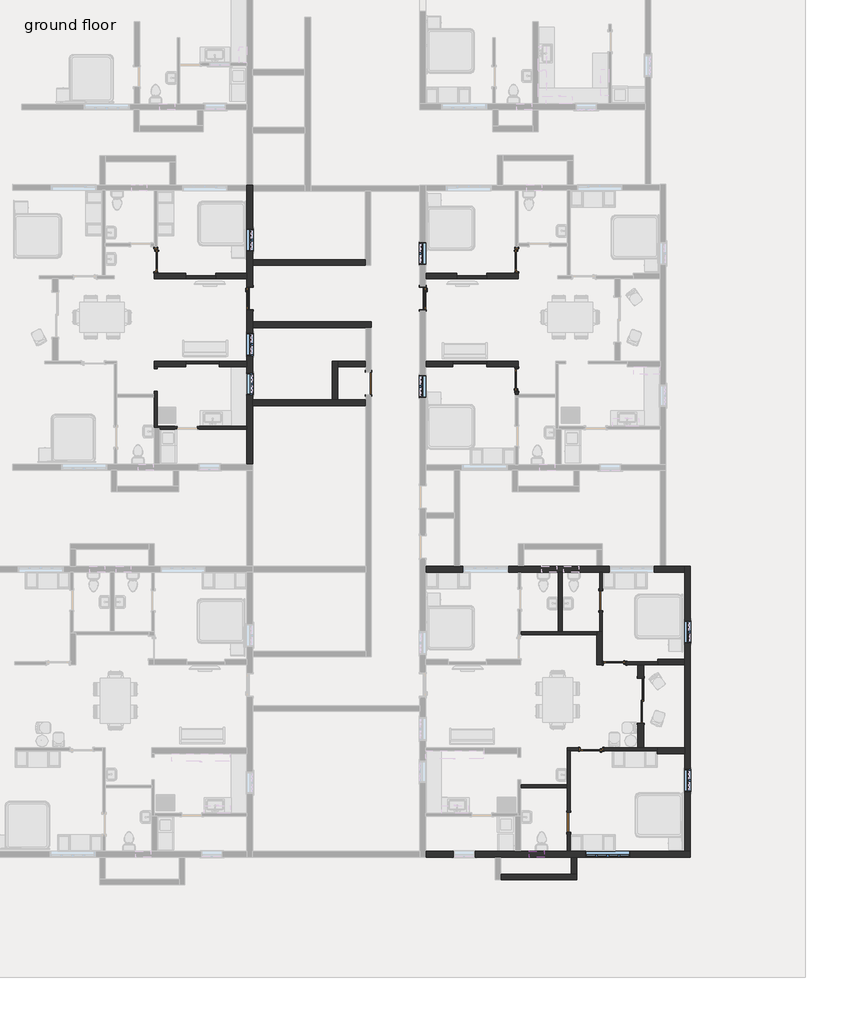
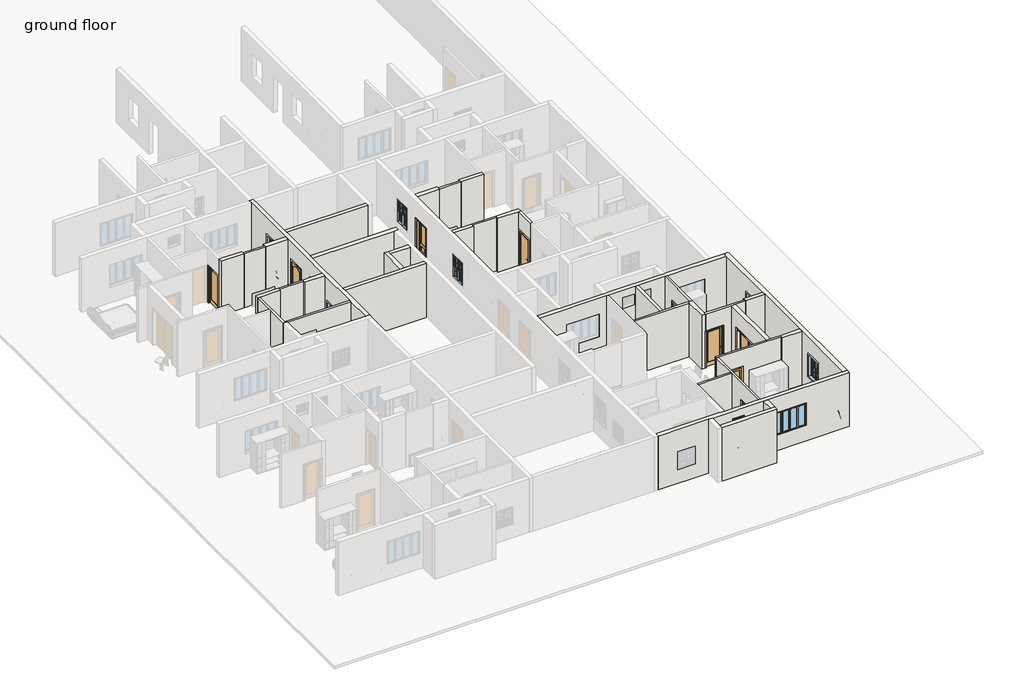
# One storey, part 3 of 16: 37 walls, 11 doors, 9 windows.
"""IFC4 building model written with IfcOpenShell, lengths in millimetres."""

from ifc_helpers import new_model, si_unit, point, frame, origin, place, context, project, spatial, polyline, ellipse_curve, trimmed, outline, extrude, faceted_brep, transform, mapped, element, save
from ifc_brep_helpers import plane_surface, extruded_surface, advanced_brep
from components import door_fe8ae985, door_f079f64e, door_d4d75d1e, door_a3feeac7, door_3c6ab76a, door_38851409, door_d141acb4, door_0ca8825f, window_ced37e8f, window_5487fb6d, window_f2d8fef0, window_45970670

model = new_model("IFC4")

# Units and contexts
model_context = context("Model", 3, world=origin())
ifc_project = project(units=[si_unit("LENGTHUNIT", "METRE", prefix="MILLI")], contexts=[model_context])

# Site, building, storey
site = spatial("IfcSite", under=ifc_project)
building = spatial("IfcBuilding", under=site)
storey = spatial("IfcBuildingStorey", under=building, Name="ground floor", Elevation=609.6)

# Doors
placement = place(None, origin())
door_shape = door_fe8ae985(model_context)
element("IfcDoor", 1, ObjectType="36\" x 84\"", at=placement, inside=storey, context=model_context, shape_type="MappedRepresentation", body=[
    mapped(door_shape, transform((59474.0062819, -2594.7113664, 609.6), x_axis=(0.0, 1.0, 0.0), y_axis=(-1.0, 0.0, 0.0), z_axis=(0.0, 0.0, 1.0))),
])
door_2_shape = door_f079f64e(model_context)
element("IfcDoor", 2, ObjectType="36\" x 84\"", at=placement, inside=storey, context=model_context, shape_type="MappedRepresentation", body=[
    mapped(door_2_shape, transform((52422.151243, -2594.7113664, 609.6), x_axis=(0.0, 1.0, 0.0), y_axis=(-1.0, 0.0, 0.0), z_axis=(0.0, 0.0, 1.0))),
])
door_3_shape = door_d4d75d1e(model_context)
element("IfcDoor", 3, ObjectType="Door-Double-Sliding : 72\" x 84\"", at=placement, inside=storey, context=model_context, shape_type="MappedRepresentation", body=[
    mapped(door_3_shape, transform((68221.1312819, -18980.3865909, 609.6), x_axis=(0.0, -1.0, 0.0), y_axis=(1.0, 0.0, 0.0), z_axis=(0.0, 0.0, 1.0))),
])
door_4_shape = door_a3feeac7(model_context)
element("IfcDoor", 4, ObjectType="Door-Interior-Single-1_Panel-Wood : 36\" x 84\"", at=placement, inside=storey, context=model_context, shape_type="MappedRepresentation", body=[
    mapped(door_4_shape, transform((63296.7062819, -1042.1363664, 609.6), x_axis=(0.0, -1.0, 0.0), y_axis=(1.0, 0.0, 0.0), z_axis=(0.0, 0.0, 1.0))),
])
element("IfcDoor", 5, ObjectType="Door-Interior-Single-1_Panel-Wood : 36\" x 84\"", at=placement, inside=storey, context=model_context, shape_type="MappedRepresentation", body=[
    mapped(door_4_shape, transform((67281.3312819, -17453.2115909, 609.6), x_axis=(-1.0, 0.0, 0.0), y_axis=(0.0, -1.0, 0.0), z_axis=(0.0, 0.0, 1.0))),
])
door_5_shape = door_3c6ab76a(model_context)
element("IfcDoor", 6, ObjectType="Door-Interior-Single-1_Panel-Wood : 36\" x 84\"", at=placement, inside=storey, context=model_context, shape_type="MappedRepresentation", body=[
    mapped(door_5_shape, transform((48599.451243, -1042.1363664, 609.6), x_axis=(0.0, -1.0, 0.0), y_axis=(1.0, 0.0, 0.0), z_axis=(0.0, 0.0, 1.0))),
])
element("IfcDoor", 7, ObjectType="Door-Interior-Single-1_Panel-Wood : 36\" x 84\"", at=placement, inside=storey, context=model_context, shape_type="MappedRepresentation", body=[
    mapped(door_5_shape, transform((63296.7062819, -5912.5863664, 609.6), x_axis=(0.0, 1.0, 0.0), y_axis=(-1.0, 0.0, 0.0), z_axis=(0.0, 0.0, 1.0))),
])
element("IfcDoor", 8, ObjectType="Door-Interior-Single-1_Panel-Wood : 36\" x 84\"", at=placement, inside=storey, context=model_context, shape_type="MappedRepresentation", body=[
    mapped(door_5_shape, transform((66335.1812819, -20964.6408586, 609.6), x_axis=(-1.0, 0.0, 0.0), y_axis=(0.0, -1.0, 0.0), z_axis=(0.0, 0.0, 1.0))),
])
door_6_shape = door_38851409(model_context)
element("IfcDoor", 9, ObjectType="Single-Flush : 32\" x 84\"", at=placement, inside=storey, context=model_context, shape_type="MappedRepresentation", body=[
    mapped(door_6_shape, transform((66728.8812819, -14903.6865909, 609.6), x_axis=(0.0, -1.0, 0.0), y_axis=(1.0, 0.0, 0.0), z_axis=(0.0, 0.0, 1.0))),
])
door_7_shape = door_d141acb4(model_context)
element("IfcDoor", 10, ObjectType="Single-Flush : 32\" x 84\"", at=placement, inside=storey, context=model_context, shape_type="MappedRepresentation", body=[
    mapped(door_7_shape, transform((65420.7812819, -23939.7365909, 609.6), x_axis=(0.0, 1.0, 0.0), y_axis=(-1.0, 0.0, 0.0), z_axis=(0.0, 0.0, 1.0))),
])
door_8_shape = door_0ca8825f(model_context)
element("IfcDoor", 11, ObjectType="Single-Flush : 36\" x 84\"", at=placement, inside=storey, context=model_context, shape_type="MappedRepresentation", body=[
    mapped(door_8_shape, transform((57261.0312819, -6052.4343195, 609.6), x_axis=(0.0, -1.0, 0.0), y_axis=(1.0, 0.0, 0.0), z_axis=(0.0, 0.0, 1.0))),
])

# Walls
element("IfcWall", 12, ObjectType="Generic - 4.5\"", at=placement, inside=storey, context=model_context, shape_type="SweptSolid", body=[
    extrude(outline(polyline([(51049.0749549, -1794.6113664), (49824.9103812, -1794.6113664), (49824.9103812, -1680.3113664), (51049.0749549, -1680.3113664), (51049.0749549, -1794.6113664)])), frame((0.0, 0.0, 609.6), z_axis=(0.0, 0.0, 1.0), x_axis=(1.0, 0.0, 0.0)), (0.0, 0.0, 1.0), 3200.4),
])
element("IfcWall", 13, ObjectType="Generic - 4.5\"", at=placement, inside=storey, context=model_context, shape_type="SweptSolid", body=[
    extrude(outline(polyline([(49809.126243, -5147.4113664), (51180.726243, -5147.4113664), (51180.726243, -5261.7113664), (49809.126243, -5261.7113664), (49809.126243, -5147.4113664)])), frame((0.0, 0.0, 609.6), z_axis=(0.0, 0.0, 1.0), x_axis=(1.0, 0.0, 0.0)), (0.0, 0.0, 1.0), 3200.4),
])
element("IfcWall", 14, ObjectType="Generic - 4.5\"", at=placement, inside=storey, context=model_context, shape_type="AdvancedBrep", body=[
    advanced_brep(
    [(48539.126243, -5376.0113664, 609.6), (48539.126243, -5455.3863664, 609.6), (48539.126243, -5455.3863664, 2540.0), (48539.126243, -6369.7863664, 2540.0), (48539.126243, -6369.7863664, 609.6), (48539.126243, -6506.3113664, 609.6), (48539.126243, -6620.6113664, 609.6), (48539.126243, -7858.8613664, 609.6), (48539.126243, -7858.8613664, 3810.0), (48539.126243, -6620.6113664, 3810.0), (48539.126243, -6506.3113664, 3810.0), (48539.126243, -5376.0113664, 3810.0), (48653.426243, -5455.3863664, 2540.0), (48653.426243, -5455.3863664, 609.6), (48653.426243, -5376.0113664, 609.6), (48653.426243, -5376.0113664, 3810.0), (48653.426243, -7801.7113664, 3810.0), (48653.426243, -7858.8613664, 3810.0), (48653.426243, -7858.8613664, 609.6), (48653.426243, -7801.7113664, 609.6), (48653.426243, -6369.7863664, 609.6), (48653.426243, -6369.7863664, 2540.0)],
    [
        (0, 1),
        (1, 2),
        (2, 3, ellipse_curve(frame((48539.126243, -5912.5863664, 2540.0), z_axis=(1.0, 0.0, 0.0), x_axis=(0.0, 1.0, 0.0)), 457.2, 203.2)),
        (3, 4),
        (4, 5),
        (5, 6),
        (6, 7),
        (7, 8),
        (8, 9),
        (9, 10),
        (10, 11),
        (11, 0),
        (12, 13),
        (13, 14),
        (14, 15),
        (15, 16),
        (16, 17),
        (17, 18),
        (18, 19),
        (19, 20),
        (20, 21),
        (21, 12, ellipse_curve(frame((48653.426243, -5912.5863664, 2540.0), z_axis=(-1.0, 0.0, 0.0), x_axis=(0.0, 1.0, 0.0)), 457.2, 203.2)),
        (13, 1),
        (0, 14),
        (18, 7),
        (4, 20),
        (17, 8),
        (15, 11),
        (2, 12),
        (21, 3),
    ],
    [
        plane_surface(frame((48539.126243, -5376.0113664, 609.6), z_axis=(-1.0, 0.0, 0.0), x_axis=(0.0, -1.0, 0.0))),
        plane_surface(frame((48653.426243, -5376.0113664, 609.6), z_axis=(1.0, 0.0, 0.0), x_axis=(0.0, 1.0, 0.0))),
        plane_surface(frame((48539.126243, -5261.7113664, 609.6), z_axis=(0.0, 0.0, -1.0), x_axis=(1.0, 0.0, 0.0))),
        plane_surface(frame((48539.126243, -7858.8613664, 609.6), z_axis=(0.0, -1.0, 0.0), x_axis=(1.0, 0.0, 0.0))),
        plane_surface(frame((48539.126243, -7858.8613664, 3810.0), z_axis=(0.0, 0.0, 1.0), x_axis=(1.0, 0.0, 0.0))),
        plane_surface(frame((48539.126243, -5376.0113664, 609.6), z_axis=(0.0, 1.0, 0.0), x_axis=(1.0, 0.0, 0.0))),
        extruded_surface(trimmed(ellipse_curve(frame((48767.726243, -5912.5863664, 2540.0), z_axis=(1.0, 0.0, 0.0), x_axis=(0.0, 1.0, 0.0)), 457.2, 203.2), [point((48767.726243, -5455.3863664, 2540.0))], [point((48767.726243, -6369.7863664, 2540.0))], True, "CARTESIAN"), (-114.29999999999563, 0.0, 0.0), 114.29999999999563),
        plane_surface(frame((48539.126243, -6369.7863664, 2540.0), z_axis=(0.0, 1.0, 0.0), x_axis=(1.0, 0.0, 0.0))),
        plane_surface(frame((48539.126243, -5455.3863664, 609.6), z_axis=(0.0, -1.0, 0.0), x_axis=(1.0, 0.0, 0.0))),
    ],
    [
        (0, [[1, 2, 3, 4, 5, 6, 7, 8, 9, 10, 11, 12]]),
        (1, [[13, 14, 15, 16, 17, 18, 19, 20, 21, 22]]),
        (2, [[-14, 23, -1, 24]]),
        (2, [[-20, -19, 25, -7, -6, -5, 26]]),
        (3, [[-8, -25, -18, 27]]),
        (4, [[-11, -10, -9, -27, -17, -16, 28]]),
        (5, [[-12, -28, -15, -24]]),
        (6, [[-3, 29, -22, 30]]),
        (7, [[-4, -30, -21, -26]]),
        (8, [[-2, -23, -13, -29]]),
    ],
),
])
element("IfcWall", 15, ObjectType="Generic - 4.5\"", at=placement, inside=storey, context=model_context, shape_type="Brep", body=[
    faceted_brep([(48767.726243, -7916.0113664, 609.6), (49466.226243, -7916.0113664, 609.6), (49466.226243, -7916.0113664, 2743.2), (50279.026243, -7916.0113664, 2743.2), (50279.026243, -7916.0113664, 609.6), (52311.026243, -7916.0113664, 609.6), (52311.026243, -7916.0113664, 3810.0), (48767.726243, -7916.0113664, 3810.0), (49466.226243, -7801.7113664, 2743.2), (49466.226243, -7801.7113664, 609.6), (48653.426243, -7801.7113664, 609.6), (48653.426243, -7801.7113664, 3810.0), (52311.026243, -7801.7113664, 3810.0), (52311.026243, -7801.7113664, 609.6), (50279.026243, -7801.7113664, 609.6), (50279.026243, -7801.7113664, 2743.2), (48767.726243, -7858.8613664, 609.6), (48653.426243, -7858.8613664, 609.6), (48653.426243, -7858.8613664, 3810.0), (48767.726243, -7858.8613664, 3810.0)], [[[0, 1, 2, 3, 4, 5, 6, 7]], [[8, 9, 10, 11, 12, 13, 14, 15]], [[14, 13, 5, 4]], [[10, 9, 1, 0, 16, 17]], [[7, 6, 12, 11, 18, 19]], [[0, 7, 19, 16]], [[19, 18, 17, 16]], [[18, 11, 10, 17]], [[6, 5, 13, 12]], [[2, 1, 9, 8]], [[3, 2, 8, 15]], [[4, 3, 15, 14]]]),
])
element("IfcWall", 16, ObjectType="Generic - 4.5\"", at=placement, inside=storey, context=model_context, shape_type="SweptSolid", body=[
    extrude(outline(polyline([(62071.2471437, -1794.6113664), (60847.08257, -1794.6113664), (60847.08257, -1680.3113664), (62071.2471437, -1680.3113664), (62071.2471437, -1794.6113664)])), frame((0.0, 0.0, 609.6), z_axis=(0.0, 0.0, 1.0), x_axis=(1.0, 0.0, 0.0)), (0.0, 0.0, 1.0), 3200.4),
])
element("IfcWall", 17, ObjectType="Generic - 4.5\"", at=placement, inside=storey, context=model_context, shape_type="SweptSolid", body=[
    extrude(outline(polyline([(60702.7312819, -5147.4113664), (62074.3312819, -5147.4113664), (62074.3312819, -5261.7113664), (60702.7312819, -5261.7113664), (60702.7312819, -5147.4113664)])), frame((0.0, 0.0, 609.6), z_axis=(0.0, 0.0, 1.0), x_axis=(1.0, 0.0, 0.0)), (0.0, 0.0, 1.0), 3200.4),
])
element("IfcWall", 18, ObjectType="Generic - 4.5\"", at=placement, inside=storey, context=model_context, shape_type="Brep", body=[
    faceted_brep([(66786.0312819, -17399.2365909, 3810.0), (69046.6312819, -17399.2365909, 3810.0), (69046.6312819, -17399.2365909, 609.6), (67763.9312819, -17399.2365909, 609.6), (67763.9312819, -17399.2365909, 2768.6), (66798.7312819, -17399.2365909, 2768.6), (66798.7312819, -17399.2365909, 609.6), (66786.0312819, -17399.2365909, 609.6), (69046.6312819, -17513.5365909, 3810.0), (68462.4312819, -17513.5365909, 3810.0), (68233.8312819, -17513.5365909, 3810.0), (66786.0312819, -17513.5365909, 3810.0), (66786.0312819, -17513.5365909, 609.6), (66798.7312819, -17513.5365909, 609.6), (66798.7312819, -17513.5365909, 2768.6), (67763.9312819, -17513.5365909, 2768.6), (67763.9312819, -17513.5365909, 609.6), (68233.8312819, -17513.5365909, 609.6), (68462.4312819, -17513.5365909, 609.6), (69046.6312819, -17513.5365909, 609.6)], [[[0, 1, 2, 3, 4, 5, 6, 7]], [[8, 9, 10, 11, 12, 13, 14, 15, 16, 17, 18, 19]], [[2, 19, 18, 17, 16, 3]], [[12, 7, 6, 13]], [[1, 0, 11, 10, 9, 8]], [[2, 1, 8, 19]], [[0, 7, 12, 11]], [[5, 14, 13, 6]], [[14, 5, 4, 15]], [[15, 4, 3, 16]]]),
])
element("IfcWall", 19, ObjectType="Generic - 4.5\"", at=placement, inside=storey, context=model_context, shape_type="Brep", body=[
    faceted_brep([(65363.6312819, -20904.3158586, 3810.0), (68233.8312819, -20904.3158586, 3810.0), (68462.4312819, -20904.3158586, 3810.0), (69021.2312819, -20904.3158586, 3810.0), (69021.2312819, -20904.3158586, 609.6), (68462.4312819, -20904.3158586, 609.6), (68233.8312819, -20904.3158586, 609.6), (66817.7812819, -20904.3158586, 609.6), (66817.7812819, -20904.3158586, 2768.6), (65852.5812819, -20904.3158586, 2768.6), (65852.5812819, -20904.3158586, 609.6), (65363.6312819, -20904.3158586, 609.6), (69021.2312819, -21018.6158586, 3810.0), (65477.9312819, -21018.6158586, 3810.0), (65363.6312819, -21018.6158586, 3810.0), (65363.6312819, -21018.6158586, 609.6), (65477.9312819, -21018.6158586, 609.6), (65852.5812819, -21018.6158586, 609.6), (65852.5812819, -21018.6158586, 2768.6), (66817.7812819, -21018.6158586, 2768.6), (66817.7812819, -21018.6158586, 609.6), (69021.2312819, -21018.6158586, 609.6)], [[[0, 1, 2, 3, 4, 5, 6, 7, 8, 9, 10, 11]], [[12, 13, 14, 15, 16, 17, 18, 19, 20, 21]], [[4, 21, 20, 7, 6, 5]], [[15, 11, 10, 17, 16]], [[3, 2, 1, 0, 14, 13, 12]], [[4, 3, 12, 21]], [[0, 11, 15, 14]], [[9, 18, 17, 10]], [[18, 9, 8, 19]], [[19, 8, 7, 20]]]),
])
element("IfcWall", 20, ObjectType="Generic - 4.5\"", at=placement, inside=storey, context=model_context, shape_type="Brep", body=[
    faceted_brep([(65363.6312819, -21018.6158586, 609.6), (65363.6312819, -22413.9790776, 609.6), (65363.6312819, -22528.2790776, 609.6), (65363.6312819, -23533.3365909, 609.6), (65363.6312819, -23533.3365909, 2743.2), (65363.6312819, -24346.1365909, 2743.2), (65363.6312819, -24346.1365909, 609.6), (65363.6312819, -25120.8365909, 609.6), (65363.6312819, -25120.8365909, 3810.0), (65363.6312819, -22528.2790776, 3810.0), (65363.6312819, -22413.9790776, 3810.0), (65363.6312819, -21018.6158586, 3810.0), (65477.9312819, -23533.3365909, 2743.2), (65477.9312819, -23533.3365909, 609.6), (65477.9312819, -21018.6158586, 609.6), (65477.9312819, -21018.6158586, 3810.0), (65477.9312819, -25120.8365909, 3810.0), (65477.9312819, -25120.8365909, 609.6), (65477.9312819, -24346.1365909, 609.6), (65477.9312819, -24346.1365909, 2743.2)], [[[0, 1, 2, 3, 4, 5, 6, 7, 8, 9, 10, 11]], [[12, 13, 14, 15, 16, 17, 18, 19]], [[18, 17, 7, 6]], [[14, 13, 3, 2, 1, 0]], [[11, 10, 9, 8, 16, 15]], [[0, 11, 15, 14]], [[8, 7, 17, 16]], [[4, 3, 13, 12]], [[5, 4, 12, 19]], [[6, 5, 19, 18]]]),
])
element("IfcWall", 21, ObjectType="Generic - 4.5\"", at=placement, inside=storey, context=model_context, shape_type="SweptSolid", body=[
    extrude(outline(polyline([(63458.6312819, -22413.9790776), (65363.6312819, -22413.9790776), (65363.6312819, -22528.2790776), (63458.6312819, -22528.2790776), (63458.6312819, -22413.9790776)])), frame((0.0, 0.0, 609.6), z_axis=(0.0, 0.0, 1.0), x_axis=(1.0, 0.0, 0.0)), (0.0, 0.0, 1.0), 3200.4),
])
element("IfcWall", 22, ObjectType="Generic - 4.5\"", at=placement, inside=storey, context=model_context, shape_type="Brep", body=[
    faceted_brep([(63471.3312819, -16294.3365909, 609.6), (66557.4312819, -16294.3365909, 609.6), (66557.4312819, -16294.3365909, 3810.0), (63471.3312819, -16294.3365909, 3810.0), (63471.3312819, -16180.0365909, 609.6), (63471.3312819, -16180.0365909, 3810.0), (64995.3312819, -16180.0365909, 3810.0), (65147.7312819, -16180.0365909, 3810.0), (66557.4312819, -16180.0365909, 3810.0), (66557.4312819, -16180.0365909, 609.6), (65147.7312819, -16180.0365909, 609.6), (64995.3312819, -16180.0365909, 609.6)], [[[0, 1, 2, 3]], [[4, 5, 6, 7, 8, 9, 10, 11]], [[1, 0, 4, 11, 10, 9]], [[3, 2, 8, 7, 6, 5]], [[2, 1, 9, 8]], [[0, 3, 5, 4]]]),
])
element("IfcWall", 23, ObjectType="Generic - 4.5\"", at=placement, inside=storey, context=model_context, shape_type="SweptSolid", body=[
    extrude(outline(polyline([(-15310.0865909, 2743.2), (-15310.0865909, 609.6), (-16180.0365909, 609.6), (-16180.0365909, 3810.0), (-13741.6365909, 3810.0), (-13741.6365909, 609.6), (-14497.2865909, 609.6), (-14497.2865909, 2743.2), (-15310.0865909, 2743.2)])), frame((66671.7312819, 0.0, 0.0), z_axis=(1.0, 0.0, 0.0), x_axis=(0.0, 1.0, 0.0)), (0.0, 0.0, 1.0), 114.3),
])
element("IfcWall", 24, ObjectType="Generic - 4.5\"", at=placement, inside=storey, context=model_context, shape_type="SweptSolid", body=[
    extrude(outline(polyline([(-6506.3113664, 3810.0), (-5376.0113664, 3810.0), (-5376.0113664, 609.6), (-5429.9863664, 609.6), (-5429.9863664, 2768.6), (-6395.1863664, 2768.6), (-6395.1863664, 609.6), (-6506.3113664, 609.6), (-6506.3113664, 3810.0)])), frame((63242.7312819, 0.0, 0.0), z_axis=(1.0, 0.0, 0.0), x_axis=(0.0, 1.0, 0.0)), (0.0, 0.0, 1.0), 114.3),
])
element("IfcWall", 25, ObjectType="Generic - 6\"", at=placement, inside=storey, context=model_context, shape_type="SweptSolid", body=[
    extrude(outline(polyline([(64995.3312819, -16180.0365909), (64995.3312819, -13741.6365909), (65147.7312819, -13741.6365909), (65147.7312819, -16180.0365909), (64995.3312819, -16180.0365909)])), frame((0.0, 0.0, 609.6), z_axis=(0.0, 0.0, 1.0), x_axis=(1.0, 0.0, 0.0)), (0.0, 0.0, 1.0), 3200.4),
])
element("IfcWall", 26, ObjectType="Generic - 9\"", at=placement, inside=storey, context=model_context, shape_type="Brep", body=[
    faceted_brep([(52539.626243, 2007.0575277, 3810.0), (52539.626243, 2006.2512916, 3810.0), (52539.626243, 1777.6512916, 3810.0), (52539.626243, -1024.9409315, 3810.0), (52539.626243, -1253.5409315, 3810.0), (52539.626243, -3551.5389812, 3810.0), (52539.626243, -3780.1389812, 3810.0), (52539.626243, -6728.8572725, 3810.0), (52539.626243, -6957.4572725, 3810.0), (52539.626243, -9357.7253443, 3810.0), (52539.626243, -9357.7253443, 609.6), (52539.626243, -6957.4572725, 609.6), (52539.626243, -6728.8572725, 609.6), (52539.626243, -3780.1389812, 609.6), (52539.626243, -3551.5389812, 609.6), (52539.626243, -3077.3113664, 609.6), (52539.626243, -3077.3113664, 2768.6), (52539.626243, -2112.1113664, 2768.6), (52539.626243, -2112.1113664, 609.6), (52539.626243, -1253.5409315, 609.6), (52539.626243, -1024.9409315, 609.6), (52539.626243, 1777.6512916, 609.6), (52539.626243, 2006.2512916, 609.6), (52539.626243, 2007.0575277, 609.6), (52539.626243, -6512.9572725, 2438.4), (52539.626243, -5649.3572725, 2438.4), (52539.626243, -5649.3572725, 1524.0), (52539.626243, -6512.9572725, 1524.0), (52539.626243, -4006.5751738, 2844.8), (52539.626243, -4006.5751738, 1524.0), (52539.626243, -4920.9751738, 1524.0), (52539.626243, -4920.9751738, 2844.8), (52539.626243, 232.3590685, 2844.8), (52539.626243, 232.3590685, 1524.0), (52539.626243, -682.0409315, 1524.0), (52539.626243, -682.0409315, 2844.8), (52311.026243, -9357.7253443, 3810.0), (52311.026243, -7916.0113664, 3810.0), (52311.026243, -7801.7113664, 3810.0), (52311.026243, -5376.0113664, 3810.0), (52311.026243, -5147.4113664, 3810.0), (52311.026243, -1794.6113664, 3810.0), (52311.026243, -1566.0113664, 3810.0), (52311.026243, 1779.3652466, 3810.0), (52311.026243, 2007.967056, 3810.0), (52311.026243, 2007.967056, 609.6), (52311.026243, 1779.3652466, 609.6), (52311.026243, -1566.0113664, 609.6), (52311.026243, -1794.6113664, 609.6), (52311.026243, -2112.1113664, 609.6), (52311.026243, -2112.1113664, 2768.6), (52311.026243, -3077.3113664, 2768.6), (52311.026243, -3077.3113664, 609.6), (52311.026243, -5147.4113664, 609.6), (52311.026243, -5376.0113664, 609.6), (52311.026243, -7801.7113664, 609.6), (52311.026243, -7916.0113664, 609.6), (52311.026243, -9357.7253443, 609.6), (52311.026243, -6512.9572725, 2438.4), (52311.026243, -6512.9572725, 1524.0), (52311.026243, -5649.3572725, 1524.0), (52311.026243, -5649.3572725, 2438.4), (52311.026243, -4006.5751738, 2844.8), (52311.026243, -4920.9751738, 2844.8), (52311.026243, -4920.9751738, 1524.0), (52311.026243, -4006.5751738, 1524.0), (52311.026243, 232.3590685, 2844.8), (52311.026243, -682.0409315, 2844.8), (52311.026243, -682.0409315, 1524.0), (52311.026243, 232.3590685, 1524.0)], [[[0, 1, 2, 3, 4, 5, 6, 7, 8, 9, 10, 11, 12, 13, 14, 15, 16, 17, 18, 19, 20, 21, 22, 23], [24, 25, 26, 27], [28, 29, 30, 31], [32, 33, 34, 35]], [[36, 37, 38, 39, 40, 41, 42, 43, 44, 45, 46, 47, 48, 49, 50, 51, 52, 53, 54, 55, 56, 57], [58, 59, 60, 61], [62, 63, 64, 65], [66, 67, 68, 69]], [[10, 57, 56, 55, 54, 53, 52, 15, 14, 13, 12, 11]], [[45, 23, 22, 21, 20, 19, 18, 49, 48, 47, 46]], [[9, 8, 7, 6, 5, 4, 3, 2, 1, 0, 44, 43, 42, 41, 40, 39, 38, 37, 36]], [[10, 9, 36, 57]], [[0, 23, 45, 44]], [[17, 50, 49, 18]], [[50, 17, 16, 51]], [[51, 16, 15, 52]], [[59, 58, 24, 27]], [[60, 59, 27, 26]], [[61, 60, 26, 25]], [[58, 61, 25, 24]], [[29, 28, 62, 65]], [[30, 29, 65, 64]], [[31, 30, 64, 63]], [[28, 31, 63, 62]], [[33, 32, 66, 69]], [[34, 33, 69, 68]], [[35, 34, 68, 67]], [[32, 35, 67, 66]]]),
])
element("IfcWall", 27, ObjectType="Generic - 9\"", at=placement, inside=storey, context=model_context, shape_type="Brep", body=[
    faceted_brep([(48539.126243, -5376.0113664, 609.6), (48653.426243, -5376.0113664, 609.6), (49809.126243, -5376.0113664, 609.6), (49809.126243, -5376.0113664, 3810.0), (48653.426243, -5376.0113664, 3810.0), (48539.126243, -5376.0113664, 3810.0), (48539.126243, -5147.4113664, 609.6), (48539.126243, -5147.4113664, 3810.0), (49809.126243, -5147.4113664, 3810.0), (49809.126243, -5147.4113664, 609.6), (49809.126243, -5261.7113664, 609.6), (49809.126243, -5261.7113664, 3810.0)], [[[0, 1, 2, 3, 4, 5]], [[6, 7, 8, 9]], [[2, 1, 0, 6, 9, 10]], [[3, 2, 10, 9, 8, 11]], [[5, 4, 3, 11, 8, 7]], [[0, 5, 7, 6]]]),
])
element("IfcWall", 28, ObjectType="Generic - 9\"", at=placement, inside=storey, context=model_context, shape_type="Brep", body=[
    faceted_brep([(51180.726243, -5376.0113664, 609.6), (52311.026243, -5376.0113664, 609.6), (52311.026243, -5376.0113664, 3810.0), (51180.726243, -5376.0113664, 3810.0), (51180.726243, -5147.4113664, 609.6), (51180.726243, -5147.4113664, 3810.0), (52311.026243, -5147.4113664, 3810.0), (52311.026243, -5147.4113664, 609.6), (51180.726243, -5261.7113664, 609.6), (51180.726243, -5261.7113664, 3810.0)], [[[0, 1, 2, 3]], [[4, 5, 6, 7]], [[1, 0, 8, 4, 7]], [[3, 2, 6, 5, 9]], [[0, 3, 9, 5, 4, 8]], [[2, 1, 7, 6]]]),
])
element("IfcWall", 29, ObjectType="Generic - 9\"", at=placement, inside=storey, context=model_context, shape_type="Brep", body=[
    faceted_brep([(48539.126243, -1794.6113664, 609.6), (49824.9103812, -1794.6113664, 609.6), (49824.9103812, -1794.6113664, 3810.0), (48539.126243, -1794.6113664, 3810.0), (48539.126243, -1566.0113664, 609.6), (48539.126243, -1566.0113664, 3810.0), (48653.426243, -1566.0113664, 3810.0), (49824.9103812, -1566.0113664, 3810.0), (49824.9103812, -1566.0113664, 609.6), (48653.426243, -1566.0113664, 609.6), (49824.9103812, -1680.3113664, 609.6), (49824.9103812, -1680.3113664, 3810.0)], [[[0, 1, 2, 3]], [[4, 5, 6, 7, 8, 9]], [[1, 0, 4, 9, 8, 10]], [[2, 1, 10, 8, 7, 11]], [[3, 2, 11, 7, 6, 5]], [[0, 3, 5, 4]]]),
])
element("IfcWall", 30, ObjectType="Generic - 9\"", at=placement, inside=storey, context=model_context, shape_type="Brep", body=[
    faceted_brep([(51049.0749549, -1794.6113664, 609.6), (52311.026243, -1794.6113664, 609.6), (52311.026243, -1794.6113664, 3810.0), (51049.0749549, -1794.6113664, 3810.0), (51049.0749549, -1566.0113664, 609.6), (51049.0749549, -1566.0113664, 3810.0), (52311.026243, -1566.0113664, 3810.0), (52311.026243, -1566.0113664, 609.6), (51049.0749549, -1680.3113664, 609.6), (51049.0749549, -1680.3113664, 3810.0)], [[[0, 1, 2, 3]], [[4, 5, 6, 7]], [[1, 0, 8, 4, 7]], [[3, 2, 6, 5, 9]], [[0, 3, 9, 5, 4, 8]], [[2, 1, 7, 6]]]),
])
element("IfcWall", 31, ObjectType="Generic - 9\"", at=placement, inside=storey, context=model_context, shape_type="Brep", body=[
    faceted_brep([(62071.2471437, -1794.6113664, 609.6), (63357.0312819, -1794.6113664, 609.6), (63357.0312819, -1794.6113664, 3810.0), (62071.2471437, -1794.6113664, 3810.0), (62071.2471437, -1566.0113664, 609.6), (62071.2471437, -1566.0113664, 3810.0), (63242.7312819, -1566.0113664, 3810.0), (63357.0312819, -1566.0113664, 3810.0), (63357.0312819, -1566.0113664, 609.6), (63242.7312819, -1566.0113664, 609.6), (62071.2471437, -1680.3113664, 609.6), (62071.2471437, -1680.3113664, 3810.0)], [[[0, 1, 2, 3]], [[4, 5, 6, 7, 8, 9]], [[1, 0, 10, 4, 9, 8]], [[3, 2, 7, 6, 5, 11]], [[0, 3, 11, 5, 4, 10]], [[2, 1, 8, 7]]]),
])
element("IfcWall", 32, ObjectType="Generic - 9\"", at=placement, inside=storey, context=model_context, shape_type="Brep", body=[
    faceted_brep([(59585.1312819, -1794.6113664, 609.6), (60847.08257, -1794.6113664, 609.6), (60847.08257, -1794.6113664, 3810.0), (59585.1312819, -1794.6113664, 3810.0), (59585.1312819, -1566.0113664, 609.6), (59585.1312819, -1566.0113664, 3810.0), (60847.08257, -1566.0113664, 3810.0), (60847.08257, -1566.0113664, 609.6), (60847.08257, -1680.3113664, 609.6), (60847.08257, -1680.3113664, 3810.0)], [[[0, 1, 2, 3]], [[4, 5, 6, 7]], [[1, 0, 4, 7, 8]], [[2, 1, 8, 7, 6, 9]], [[3, 2, 9, 6, 5]], [[0, 3, 5, 4]]]),
])
element("IfcWall", 33, ObjectType="Generic - 9\"", at=placement, inside=storey, context=model_context, shape_type="Brep", body=[
    faceted_brep([(59585.1312819, -5376.0113664, 609.6), (60702.7312819, -5376.0113664, 609.6), (60702.7312819, -5376.0113664, 3810.0), (59585.1312819, -5376.0113664, 3810.0), (59585.1312819, -5147.4113664, 609.6), (59585.1312819, -5147.4113664, 3810.0), (60702.7312819, -5147.4113664, 3810.0), (60702.7312819, -5147.4113664, 609.6), (60702.7312819, -5261.7113664, 609.6), (60702.7312819, -5261.7113664, 3810.0)], [[[0, 1, 2, 3]], [[4, 5, 6, 7]], [[1, 0, 4, 7, 8]], [[2, 1, 8, 7, 6, 9]], [[3, 2, 9, 6, 5]], [[0, 3, 5, 4]]]),
])
element("IfcWall", 34, ObjectType="Generic - 9\"", at=placement, inside=storey, context=model_context, shape_type="Brep", body=[
    faceted_brep([(62074.3312819, -5376.0113664, 609.6), (63242.7312819, -5376.0113664, 609.6), (63357.0312819, -5376.0113664, 609.6), (63357.0312819, -5376.0113664, 3810.0), (63242.7312819, -5376.0113664, 3810.0), (62074.3312819, -5376.0113664, 3810.0), (62074.3312819, -5147.4113664, 609.6), (62074.3312819, -5147.4113664, 3810.0), (63357.0312819, -5147.4113664, 3810.0), (63357.0312819, -5147.4113664, 609.6), (62074.3312819, -5261.7113664, 609.6), (62074.3312819, -5261.7113664, 3810.0)], [[[0, 1, 2, 3, 4, 5]], [[6, 7, 8, 9]], [[2, 1, 0, 10, 6, 9]], [[5, 4, 3, 8, 7, 11]], [[0, 5, 11, 7, 6, 10]], [[3, 2, 9, 8]]]),
])
element("IfcWall", 35, ObjectType="Generic - 9\"", at=placement, inside=storey, context=model_context, shape_type="Brep", body=[
    faceted_brep([(59585.1312819, -25349.4365909, 609.6), (62419.2921849, -25349.4365909, 609.6), (62647.8921849, -25349.4365909, 609.6), (65521.3932249, -25349.4365909, 609.6), (65749.9932249, -25349.4365909, 609.6), (70367.4312819, -25349.4365909, 609.6), (70367.4312819, -25349.4365909, 3810.0), (65749.9932249, -25349.4365909, 3810.0), (65521.3932249, -25349.4365909, 3810.0), (62647.8921849, -25349.4365909, 3810.0), (62419.2921849, -25349.4365909, 3810.0), (59585.1312819, -25349.4365909, 3810.0), (66092.8932249, -25349.4365909, 2870.2), (67921.6932249, -25349.4365909, 2870.2), (67921.6932249, -25349.4365909, 1524.0), (66092.8932249, -25349.4365909, 1524.0), (60730.1921849, -25349.4365909, 2438.4), (61593.7921849, -25349.4365909, 2438.4), (61593.7921849, -25349.4365909, 1524.0), (60730.1921849, -25349.4365909, 1524.0), (64411.1312819, -25349.4365909, 3352.8), (64411.1312819, -25349.4365909, 2743.2), (63801.5312819, -25349.4365909, 2743.2), (63801.5312819, -25349.4365909, 3352.8), (59585.1312819, -25120.8365909, 609.6), (59585.1312819, -25120.8365909, 3810.0), (63230.0312819, -25120.8365909, 3810.0), (63458.6312819, -25120.8365909, 3810.0), (65363.6312819, -25120.8365909, 3810.0), (65477.9312819, -25120.8365909, 3810.0), (70138.8312819, -25120.8365909, 3810.0), (70367.4312819, -25120.8365909, 3810.0), (70367.4312819, -25120.8365909, 609.6), (70138.8312819, -25120.8365909, 609.6), (65477.9312819, -25120.8365909, 609.6), (65363.6312819, -25120.8365909, 609.6), (63458.6312819, -25120.8365909, 609.6), (63230.0312819, -25120.8365909, 609.6), (66092.8932249, -25120.8365909, 2870.2), (66092.8932249, -25120.8365909, 1524.0), (67921.6932249, -25120.8365909, 1524.0), (67921.6932249, -25120.8365909, 2870.2), (60730.1921849, -25120.8365909, 2438.4), (60730.1921849, -25120.8365909, 1524.0), (61593.7921849, -25120.8365909, 1524.0), (61593.7921849, -25120.8365909, 2438.4), (64411.1312819, -25120.8365909, 3352.8), (63801.5312819, -25120.8365909, 3352.8), (63801.5312819, -25120.8365909, 2743.2), (64411.1312819, -25120.8365909, 2743.2)], [[[0, 1, 2, 3, 4, 5, 6, 7, 8, 9, 10, 11], [12, 13, 14, 15], [16, 17, 18, 19], [20, 21, 22, 23]], [[24, 25, 26, 27, 28, 29, 30, 31, 32, 33, 34, 35, 36, 37], [38, 39, 40, 41], [42, 43, 44, 45], [46, 47, 48, 49]], [[5, 4, 3, 2, 1, 0, 24, 37, 36, 35, 34, 33, 32]], [[11, 10, 9, 8, 7, 6, 31, 30, 29, 28, 27, 26, 25]], [[0, 11, 25, 24]], [[6, 5, 32, 31]], [[39, 38, 12, 15]], [[40, 39, 15, 14]], [[41, 40, 14, 13]], [[38, 41, 13, 12]], [[43, 42, 16, 19]], [[44, 43, 19, 18]], [[45, 44, 18, 17]], [[42, 45, 17, 16]], [[21, 20, 46, 49]], [[22, 21, 49, 48]], [[23, 22, 48, 47]], [[20, 23, 47, 46]]]),
])
element("IfcWall", 36, ObjectType="Generic - 9\"", at=placement, inside=storey, context=model_context, shape_type="Brep", body=[
    faceted_brep([(70367.4312819, -25120.8365909, 609.6), (70367.4312819, -13513.0365909, 609.6), (70367.4312819, -13513.0365909, 3810.0), (70367.4312819, -25120.8365909, 3810.0), (70367.4312819, -21780.6158586, 2844.8), (70367.4312819, -21780.6158586, 1524.0), (70367.4312819, -22695.0158586, 1524.0), (70367.4312819, -22695.0158586, 2844.8), (70367.4312819, -15722.8365909, 2844.8), (70367.4312819, -15722.8365909, 1524.0), (70367.4312819, -16637.2365909, 1524.0), (70367.4312819, -16637.2365909, 2844.8), (70138.8312819, -25120.8365909, 609.6), (70138.8312819, -25120.8365909, 3810.0), (70138.8312819, -21132.9158586, 3810.0), (70138.8312819, -20904.3158586, 3810.0), (70138.8312819, -17513.5365909, 3810.0), (70138.8312819, -17284.9365909, 3810.0), (70138.8312819, -13741.6365909, 3810.0), (70138.8312819, -13513.0365909, 3810.0), (70138.8312819, -13513.0365909, 609.6), (70138.8312819, -13741.6365909, 609.6), (70138.8312819, -17284.9365909, 609.6), (70138.8312819, -17513.5365909, 609.6), (70138.8312819, -20904.3158586, 609.6), (70138.8312819, -21132.9158586, 609.6), (70138.8312819, -21780.6158586, 2844.8), (70138.8312819, -22695.0158586, 2844.8), (70138.8312819, -22695.0158586, 1524.0), (70138.8312819, -21780.6158586, 1524.0), (70138.8312819, -15722.8365909, 2844.8), (70138.8312819, -16637.2365909, 2844.8), (70138.8312819, -16637.2365909, 1524.0), (70138.8312819, -15722.8365909, 1524.0)], [[[0, 1, 2, 3], [4, 5, 6, 7], [8, 9, 10, 11]], [[12, 13, 14, 15, 16, 17, 18, 19, 20, 21, 22, 23, 24, 25], [26, 27, 28, 29], [30, 31, 32, 33]], [[1, 0, 12, 25, 24, 23, 22, 21, 20]], [[3, 2, 19, 18, 17, 16, 15, 14, 13]], [[0, 3, 13, 12]], [[2, 1, 20, 19]], [[5, 4, 26, 29]], [[6, 5, 29, 28]], [[7, 6, 28, 27]], [[4, 7, 27, 26]], [[9, 8, 30, 33]], [[10, 9, 33, 32]], [[11, 10, 32, 31]], [[8, 11, 31, 30]]]),
])
element("IfcWall", 37, ObjectType="Generic - 9\"", at=placement, inside=storey, context=model_context, shape_type="Brep", body=[
    faceted_brep([(70138.8312819, -13513.0365909, 609.6), (69364.1312819, -13513.0365909, 609.6), (69135.5312819, -13513.0365909, 609.6), (66786.0312819, -13513.0365909, 609.6), (66557.4312819, -13513.0365909, 609.6), (63585.6312819, -13513.0365909, 609.6), (63357.0312819, -13513.0365909, 609.6), (60979.6016338, -13513.0365909, 609.6), (60751.0016338, -13513.0365909, 609.6), (59585.1312819, -13513.0365909, 609.6), (59585.1312819, -13513.0365909, 3810.0), (60751.0016338, -13513.0365909, 3810.0), (60979.6016338, -13513.0365909, 3810.0), (63357.0312819, -13513.0365909, 3810.0), (63585.6312819, -13513.0365909, 3810.0), (66557.4312819, -13513.0365909, 3810.0), (66786.0312819, -13513.0365909, 3810.0), (69135.5312819, -13513.0365909, 3810.0), (69364.1312819, -13513.0365909, 3810.0), (70138.8312819, -13513.0365909, 3810.0), (62956.9812819, -13513.0365909, 2870.2), (61128.1812819, -13513.0365909, 2870.2), (61128.1812819, -13513.0365909, 1524.0), (62956.9812819, -13513.0365909, 1524.0), (68903.7562819, -13513.0365909, 2870.2), (67074.9562819, -13513.0365909, 2870.2), (67074.9562819, -13513.0365909, 1524.0), (68903.7562819, -13513.0365909, 1524.0), (65223.9312819, -13513.0365909, 3352.8), (65223.9312819, -13513.0365909, 2743.2), (65833.5312819, -13513.0365909, 2743.2), (65833.5312819, -13513.0365909, 3352.8), (64309.5312819, -13513.0365909, 3352.8), (64309.5312819, -13513.0365909, 2743.2), (64919.1312819, -13513.0365909, 2743.2), (64919.1312819, -13513.0365909, 3352.8), (70138.8312819, -13741.6365909, 609.6), (70138.8312819, -13741.6365909, 3810.0), (66786.0312819, -13741.6365909, 3810.0), (66671.7312819, -13741.6365909, 3810.0), (65147.7312819, -13741.6365909, 3810.0), (64995.3312819, -13741.6365909, 3810.0), (63471.3312819, -13741.6365909, 3810.0), (63357.0312819, -13741.6365909, 3810.0), (59585.1312819, -13741.6365909, 3810.0), (59585.1312819, -13741.6365909, 609.6), (63357.0312819, -13741.6365909, 609.6), (63471.3312819, -13741.6365909, 609.6), (64995.3312819, -13741.6365909, 609.6), (65147.7312819, -13741.6365909, 609.6), (66671.7312819, -13741.6365909, 609.6), (66786.0312819, -13741.6365909, 609.6), (62956.9812819, -13741.6365909, 2870.2), (62956.9812819, -13741.6365909, 1524.0), (61128.1812819, -13741.6365909, 1524.0), (61128.1812819, -13741.6365909, 2870.2), (68903.7562819, -13741.6365909, 2870.2), (68903.7562819, -13741.6365909, 1524.0), (67074.9562819, -13741.6365909, 1524.0), (67074.9562819, -13741.6365909, 2870.2), (65223.9312819, -13741.6365909, 3352.8), (65833.5312819, -13741.6365909, 3352.8), (65833.5312819, -13741.6365909, 2743.2), (65223.9312819, -13741.6365909, 2743.2), (64309.5312819, -13741.6365909, 3352.8), (64919.1312819, -13741.6365909, 3352.8), (64919.1312819, -13741.6365909, 2743.2), (64309.5312819, -13741.6365909, 2743.2)], [[[0, 1, 2, 3, 4, 5, 6, 7, 8, 9, 10, 11, 12, 13, 14, 15, 16, 17, 18, 19], [20, 21, 22, 23], [24, 25, 26, 27], [28, 29, 30, 31], [32, 33, 34, 35]], [[36, 37, 38, 39, 40, 41, 42, 43, 44, 45, 46, 47, 48, 49, 50, 51], [52, 53, 54, 55], [56, 57, 58, 59], [60, 61, 62, 63], [64, 65, 66, 67]], [[9, 8, 7, 6, 5, 4, 3, 2, 1, 0, 36, 51, 50, 49, 48, 47, 46, 45]], [[19, 18, 17, 16, 15, 14, 13, 12, 11, 10, 44, 43, 42, 41, 40, 39, 38, 37]], [[0, 19, 37, 36]], [[10, 9, 45, 44]], [[53, 52, 20, 23]], [[54, 53, 23, 22]], [[55, 54, 22, 21]], [[52, 55, 21, 20]], [[57, 56, 24, 27]], [[58, 57, 27, 26]], [[59, 58, 26, 25]], [[56, 59, 25, 24]], [[29, 28, 60, 63]], [[30, 29, 63, 62]], [[31, 30, 62, 61]], [[28, 31, 61, 60]], [[33, 32, 64, 67]], [[34, 33, 67, 66]], [[35, 34, 66, 65]], [[32, 35, 65, 64]]]),
])
element("IfcWall", 38, ObjectType="Generic - 9\"", at=placement, inside=storey, context=model_context, shape_type="Brep", body=[
    faceted_brep([(66786.0312819, -17513.5365909, 609.6), (66786.0312819, -17399.2365909, 609.6), (66786.0312819, -16180.0365909, 609.6), (66786.0312819, -16180.0365909, 3810.0), (66786.0312819, -17399.2365909, 3810.0), (66786.0312819, -17513.5365909, 3810.0), (66557.4312819, -17513.5365909, 609.6), (66557.4312819, -17513.5365909, 3810.0), (66557.4312819, -16294.3365909, 3810.0), (66557.4312819, -16180.0365909, 3810.0), (66557.4312819, -16180.0365909, 609.6), (66557.4312819, -16294.3365909, 609.6), (66671.7312819, -16180.0365909, 609.6), (66671.7312819, -16180.0365909, 3810.0)], [[[0, 1, 2, 3, 4, 5]], [[6, 7, 8, 9, 10, 11]], [[2, 1, 0, 6, 11, 10, 12]], [[5, 4, 3, 13, 9, 8, 7]], [[0, 5, 7, 6]], [[3, 2, 12, 10, 9, 13]]]),
])
element("IfcWall", 39, ObjectType="Generic - 9\"", at=placement, inside=storey, context=model_context, shape_type="Brep", body=[
    faceted_brep([(70138.8312819, -17284.9365909, 609.6), (69046.6312819, -17284.9365909, 609.6), (69046.6312819, -17284.9365909, 3810.0), (70138.8312819, -17284.9365909, 3810.0), (70138.8312819, -17513.5365909, 609.6), (70138.8312819, -17513.5365909, 3810.0), (69046.6312819, -17513.5365909, 3810.0), (69046.6312819, -17513.5365909, 609.6), (69046.6312819, -17399.2365909, 609.6), (69046.6312819, -17399.2365909, 3810.0)], [[[0, 1, 2, 3]], [[4, 5, 6, 7]], [[1, 0, 4, 7, 8]], [[2, 1, 8, 7, 6, 9]], [[3, 2, 9, 6, 5]], [[0, 3, 5, 4]]]),
])
element("IfcWall", 40, ObjectType="Generic - 9\"", at=placement, inside=storey, context=model_context, shape_type="Brep", body=[
    faceted_brep([(70138.8312819, -20904.3158586, 609.6), (69021.2312819, -20904.3158586, 609.6), (69021.2312819, -20904.3158586, 3810.0), (70138.8312819, -20904.3158586, 3810.0), (70138.8312819, -21132.9158586, 609.6), (70138.8312819, -21132.9158586, 3810.0), (69021.2312819, -21132.9158586, 3810.0), (69021.2312819, -21132.9158586, 609.6), (69021.2312819, -21018.6158586, 609.6), (69021.2312819, -21018.6158586, 3810.0)], [[[0, 1, 2, 3]], [[4, 5, 6, 7]], [[1, 0, 4, 7, 8]], [[2, 1, 8, 7, 6, 9]], [[3, 2, 9, 6, 5]], [[0, 3, 5, 4]]]),
])
element("IfcWall", 41, ObjectType="Generic - 9\"", at=placement, inside=storey, context=model_context, shape_type="SweptSolid", body=[
    extrude(outline(polyline([(-19894.7865909, 2743.2), (-19894.7865909, 609.6), (-20904.3158586, 609.6), (-20904.3158586, 3810.0), (-17513.5365909, 3810.0), (-17513.5365909, 609.6), (-18065.9865909, 609.6), (-18065.9865909, 2743.2), (-19894.7865909, 2743.2)])), frame((68233.8312819, 0.0, 0.0), z_axis=(1.0, 0.0, 0.0), x_axis=(0.0, 1.0, 0.0)), (0.0, 0.0, 1.0), 228.6),
])
element("IfcWall", 42, ObjectType="Generic - 9\"", at=placement, inside=storey, context=model_context, shape_type="Brep", body=[
    faceted_brep([(62647.8921849, -26271.1649893, 609.6), (65749.9932249, -26271.1649893, 609.6), (65749.9932249, -26271.1649893, 3810.0), (62647.8921849, -26271.1649893, 3810.0), (62647.8921849, -26042.5649893, 609.6), (62647.8921849, -26042.5649893, 3810.0), (65521.3932249, -26042.5649893, 3810.0), (65749.9932249, -26042.5649893, 3810.0), (65749.9932249, -26042.5649893, 609.6), (65521.3932249, -26042.5649893, 609.6)], [[[0, 1, 2, 3]], [[4, 5, 6, 7, 8, 9]], [[1, 0, 4, 9, 8]], [[3, 2, 7, 6, 5]], [[0, 3, 5, 4]], [[2, 1, 8, 7]]]),
])
element("IfcWall", 43, ObjectType="Generic - 9\"", at=placement, inside=storey, context=model_context, shape_type="SweptSolid", body=[
    extrude(outline(polyline([(65749.9932249, -25349.4365909), (65749.9932249, -26042.5649893), (65521.3932249, -26042.5649893), (65521.3932249, -25349.4365909), (65749.9932249, -25349.4365909)])), frame((0.0, 0.0, 609.6), z_axis=(0.0, 0.0, 1.0), x_axis=(1.0, 0.0, 0.0)), (0.0, 0.0, 1.0), 3200.4),
])
element("IfcWall", 44, ObjectType="Generic - 9\"", at=placement, inside=storey, context=model_context, shape_type="SweptSolid", body=[
    extrude(outline(polyline([(52539.626243, -1024.9409315), (57134.0312819, -1024.9409315), (57134.0312819, -1253.5409315), (52539.626243, -1253.5409315), (52539.626243, -1024.9409315)])), frame((0.0, 0.0, 609.6), z_axis=(0.0, 0.0, 1.0), x_axis=(1.0, 0.0, 0.0)), (0.0, 0.0, 1.0), 3200.4),
])
element("IfcWall", 45, ObjectType="Generic - 9\"", at=placement, inside=storey, context=model_context, shape_type="Brep", body=[
    faceted_brep([(52539.626243, -3780.1389812, 609.6), (57146.7312819, -3780.1389812, 609.6), (57375.3312819, -3780.1389812, 609.6), (57375.3312819, -3780.1389812, 3810.0), (57146.7312819, -3780.1389812, 3810.0), (52539.626243, -3780.1389812, 3810.0), (52539.626243, -3551.5389812, 609.6), (52539.626243, -3551.5389812, 3810.0), (57375.3312819, -3551.5389812, 3810.0), (57375.3312819, -3551.5389812, 609.6)], [[[0, 1, 2, 3, 4, 5]], [[6, 7, 8, 9]], [[2, 1, 0, 6, 9]], [[5, 4, 3, 8, 7]], [[0, 5, 7, 6]], [[3, 2, 9, 8]]]),
])
element("IfcWall", 46, ObjectType="Generic - 9\"", at=placement, inside=storey, context=model_context, shape_type="Brep", body=[
    faceted_brep([(57146.7312819, -6728.8572725, 609.6), (56016.4312819, -6728.8572725, 609.6), (55787.8312819, -6728.8572725, 609.6), (52539.626243, -6728.8572725, 609.6), (52539.626243, -6728.8572725, 3810.0), (55787.8312819, -6728.8572725, 3810.0), (56016.4312819, -6728.8572725, 3810.0), (57146.7312819, -6728.8572725, 3810.0), (57146.7312819, -6957.4572725, 609.6), (57146.7312819, -6957.4572725, 3810.0), (52539.626243, -6957.4572725, 3810.0), (52539.626243, -6957.4572725, 609.6)], [[[0, 1, 2, 3, 4, 5, 6, 7]], [[8, 9, 10, 11]], [[3, 2, 1, 0, 8, 11]], [[7, 6, 5, 4, 10, 9]], [[0, 7, 9, 8]], [[4, 3, 11, 10]]]),
])
element("IfcWall", 47, ObjectType="Generic - 9\"", at=placement, inside=storey, context=model_context, shape_type="Brep", body=[
    faceted_brep([(56016.4312819, -6728.8572725, 609.6), (56016.4312819, -5376.0113664, 609.6), (56016.4312819, -5147.4113664, 609.6), (56016.4312819, -5147.4113664, 3810.0), (56016.4312819, -5376.0113664, 3810.0), (56016.4312819, -6728.8572725, 3810.0), (55787.8312819, -6728.8572725, 609.6), (55787.8312819, -6728.8572725, 3810.0), (55787.8312819, -5147.4113664, 3810.0), (55787.8312819, -5147.4113664, 609.6)], [[[0, 1, 2, 3, 4, 5]], [[6, 7, 8, 9]], [[2, 1, 0, 6, 9]], [[5, 4, 3, 8, 7]], [[0, 5, 7, 6]], [[3, 2, 9, 8]]]),
])
element("IfcWall", 48, ObjectType="Generic - 9\"", at=placement, inside=storey, context=model_context, shape_type="SweptSolid", body=[
    extrude(outline(polyline([(57146.7312819, -5376.0113664), (56016.4312819, -5376.0113664), (56016.4312819, -5147.4113664), (57146.7312819, -5147.4113664), (57146.7312819, -5376.0113664)])), frame((0.0, 0.0, 609.6), z_axis=(0.0, 0.0, 1.0), x_axis=(1.0, 0.0, 0.0)), (0.0, 0.0, 1.0), 3200.4),
])

# Windows
window_shape = window_ced37e8f(model_context)
element("IfcWindow", 49, ObjectType="Window-Casement-Double-Awning : 34\" x 36\"", at=placement, inside=storey, context=model_context, shape_type="MappedRepresentation", body=[
    mapped(window_shape, transform((52425.326243, -6081.1572725, 609.6), x_axis=(0.0, -1.0, 0.0), y_axis=(1.0, 0.0, 0.0), z_axis=(0.0, 0.0, 1.0))),
])
window_2_shape = window_5487fb6d(model_context)
element("IfcWindow", 50, ObjectType="Window-Casement-Multi-Sash-Horizontal : 72\" x 53\"", at=placement, inside=storey, context=model_context, shape_type="MappedRepresentation", body=[
    mapped(window_2_shape, transform((67007.2932249, -25235.1365909, 609.6), x_axis=(-1.0, 0.0, 0.0), y_axis=(0.0, -1.0, 0.0), z_axis=(0.0, 0.0, 1.0))),
])
window_3_shape = window_f2d8fef0(model_context)
element("IfcWindow", 51, ObjectType="Window-Louvers : 24\" x 24\"", at=placement, inside=storey, context=model_context, shape_type="MappedRepresentation", body=[
    mapped(window_3_shape, transform((64106.3312819, -25241.4865909, 1828.8), x_axis=(-1.0, 0.0, 0.0), y_axis=(0.0, -1.0, 0.0), z_axis=(0.0, 0.0, 1.0))),
])
window_4_shape = window_45970670(model_context)
element("IfcWindow", 52, ObjectType="Window-Single-Hung-Double : 36\" x 52\"", at=placement, inside=storey, context=model_context, shape_type="MappedRepresentation", body=[
    mapped(window_4_shape, transform((59470.8312819, -6176.1113664, 609.6), x_axis=(0.0, 1.0, 0.0), y_axis=(-1.0, 0.0, 0.0), z_axis=(0.0, 0.0, 1.0))),
])
element("IfcWindow", 53, ObjectType="Window-Single-Hung-Double : 36\" x 52\"", at=placement, inside=storey, context=model_context, shape_type="MappedRepresentation", body=[
    mapped(window_4_shape, transform((70253.1312819, -22237.8158586, 609.6), x_axis=(0.0, -1.0, 0.0), y_axis=(1.0, 0.0, 0.0), z_axis=(0.0, 0.0, 1.0))),
])
element("IfcWindow", 54, ObjectType="Window-Single-Hung-Double : 36\" x 52\"", at=placement, inside=storey, context=model_context, shape_type="MappedRepresentation", body=[
    mapped(window_4_shape, transform((70253.1312819, -16180.0365909, 609.6), x_axis=(0.0, -1.0, 0.0), y_axis=(1.0, 0.0, 0.0), z_axis=(0.0, 0.0, 1.0))),
])
element("IfcWindow", 55, ObjectType="Window-Single-Hung-Double : 36\" x 52\"", at=placement, inside=storey, context=model_context, shape_type="MappedRepresentation", body=[
    mapped(window_4_shape, transform((59470.8312819, -765.9113664, 609.6), x_axis=(0.0, 1.0, 0.0), y_axis=(-1.0, 0.0, 0.0), z_axis=(0.0, 0.0, 1.0))),
])
element("IfcWindow", 56, ObjectType="Window-Single-Hung-Double : 36\" x 52\"", at=placement, inside=storey, context=model_context, shape_type="MappedRepresentation", body=[
    mapped(window_4_shape, transform((52425.326243, -4463.7751738, 609.6), x_axis=(0.0, -1.0, 0.0), y_axis=(1.0, 0.0, 0.0), z_axis=(0.0, 0.0, 1.0))),
])
element("IfcWindow", 57, ObjectType="Window-Single-Hung-Double : 36\" x 52\"", at=placement, inside=storey, context=model_context, shape_type="MappedRepresentation", body=[
    mapped(window_4_shape, transform((52425.326243, -224.8409315, 609.6), x_axis=(0.0, -1.0, 0.0), y_axis=(1.0, 0.0, 0.0), z_axis=(0.0, 0.0, 1.0))),
])

save(model, "model.ifc")

# Revit data of these elements
# Type "36\" x 84\""
#   Type Mark = "11"
#   Assembly Code = "B2030100"
#   Analytic Construction = "French door, wood frame with single glass"
#   Threshold Offset [instance default] = 0' - 0 1/2"
#   Thickness = 0' - 1 3/8"
#   Thermal Resistance (R) = 1.0696 (h·ft²·°F)/BTU
#   Swing Angle [instance default] = 90.00°
#   Stiles = 0' - 4 3/4"
#   Rough Width = 3' - 2"
#   Rough Height = 7' - 1"
#   Radius = 1' - 8.05625"
#   Lock Rail = 0' - 7 1/8"
#   Height = 7' - 0"
#   Width = 3' - 0"
#   Heat Transfer Coefficient (U) = 0.9350 BTU/(h·ft²·°F)
#   Door Offset [instance default] = 0' - 0"
#   Bottom Rail = 0' - 9 1/2"
#   Threshold [instance default] = yes
#   Function = 1
#   Exterior Trim [instance default] = yes
#   Trim Material = Cherry
#   Threshold Material = Cherry
#   Panel Material = Cherry
#   Glazing = Glass
#   Frame Material = Cherry
#   Door Handle Material = Aluminum
#   Visual Light Transmittance = 0
#   Solar Heat Gain Coefficient = 0
#   Wall Closure = (empty or 0)
#   Construction Type = (empty or 0)
# Type "Door-Double-Sliding : 72\" x 84\""
#   Type Mark = "12"
#   Construction Type Id = "opn-d45"
#   Assembly Code = "C1020"
#   Analytic Construction = "Wood frame, double glass door "
#   Thickness = 0' - 2"
#   Thermal Resistance (R) = 1.8150 (h·ft²·°F)/BTU
#   Heat Transfer Coefficient (U) = 0.5510 BTU/(h·ft²·°F)
#   Height = 7' - 0"
#   Rail Width = 0' - 2"
#   Stiles = 0' - 2"
#   Trim Projection Ext = 0' - 1"
#   Trim Projection Int = 0' - 1"
#   Trim Width = 0' - 3"
#   Width = 6' - 0"
#   Define Thermal Properties by = 1
#   Glazing = Glass
#   Panel Material = Wood - Birch - Solid Stained Light Low Gloss
#   Trim Material = Paint - Sienna
#   Visual Light Transmittance = 0
#   Solar Heat Gain Coefficient = 0
#   Function = (empty or 0)
#   Wall Closure = (empty or 0)
# Type "Door-Interior-Single-1_Panel-Wood : 36\" x 84\""
#   Type Mark = "8"
#   Assembly Code = "C1020300"
#   Analytic Construction = "Wooden"
#   Top Rail = 0' - 4 11/16"
#   Thickness = 0' - 1 3/8"
#   Thermal Resistance (R) = 2.5876 (h·ft²·°F)/BTU
#   Swing Angle [instance default] = 90.00°
#   Stiles = 0' - 4 3/4"
#   Rough Width = 3' - 2"
#   Rough Height = 7' - 1"
#   Height = 7' - 0"
#   Width = 3' - 0"
#   Heat Transfer Coefficient (U) = 0.3865 BTU/(h·ft²·°F)
#   Bottom Rail = 0' - 9 1/8"
#   Trim Material = Cherry
#   Panel Material = Cherry
#   Frame Material = Cherry
#   Door Handle Material = Aluminum
#   Visual Light Transmittance = 0
#   Solar Heat Gain Coefficient = 0
#   Wall Closure = (empty or 0)
#   Function = (empty or 0)
# Type "Single-Flush : 32\" x 84\""
#   Type Mark = "3"
#   Construction Type Id = "MDOOR"
#   Assembly Code = "C1020"
#   Analytic Construction = "Metal"
#   Thickness = 0' - 2"
#   Heat Transfer Coefficient (U) = 0.651978 BTU/(h·ft²·°F)
#   Height = 7' - 0"
#   Trim Projection Ext = 0' - 1"
#   Trim Projection Int = 0' - 1"
#   Trim Width = 0' - 3"
#   Width = 2' - 8"
#   Define Thermal Properties by = 1
#   Define Thermal Properties by = 1
#   Door Material = Door - Panel
#   Frame Material = Door - Frame
#   Visual Light Transmittance = 0
#   Solar Heat Gain Coefficient = 0
#   Function = (empty or 0)
#   Wall Closure = (empty or 0)
# Type "Single-Flush : 36\" x 84\""
#   Type Mark = "1"
#   Construction Type Id = "MDOOR"
#   Assembly Code = "C1020"
#   Analytic Construction = "Metal"
#   Thickness = 0' - 2"
#   Heat Transfer Coefficient (U) = 0.651978 BTU/(h·ft²·°F)
#   Height = 7' - 0"
#   Trim Projection Ext = 0' - 1"
#   Trim Projection Int = 0' - 1"
#   Trim Width = 0' - 3"
#   Width = 3' - 0"
#   Define Thermal Properties by = 1
#   Define Thermal Properties by = 1
#   Door Material = Door - Panel
#   Frame Material = Door - Frame
#   Visual Light Transmittance = 0
#   Solar Heat Gain Coefficient = 0
#   Function = (empty or 0)
#   Wall Closure = (empty or 0)
# Type "Generic - 4.5\""
#   Assembly Code = "B2010"
#   Layers, outside or top first: 0' - 4 1/2" no material (function 1)
# Type "Generic - 6\""
#   Assembly Code = "B2010"
#   Layers, outside or top first: 0' - 6" no material (function 1)
# Type "Generic - 9\""
#   Assembly Code = "B2010"
#   Layers, outside or top first: 0' - 9" no material (function 1)
# Type "Window-Casement-Double-Awning : 34\" x 36\""
#   Type Mark = "28"
#   Fire Rating = "0.5h"
#   Assembly Code = "B2020100"
#   Analytic Construction = "Double glazing - domestic"
#   Window Inset [instance default] = 0' - 0"
#   Wall Thickness [instance default] = 0' - 6"
#   Interior Wall Closure [instance default] = 0' - 2 1/4"
#   Half Width = 1' - 5"
#   Visual Light Transmittance = 0.81
#   Thermal Resistance (R) = 1.8146 (h·ft²·°F)/BTU
#   Solar Heat Gain Coefficient = 0.76
#   Rough Width = 2' - 10 1/2"
#   Rough Height = 3' - 0 1/2"
#   Open Window Height = 2' - 0"
#   Height = 3' - 0"
#   Heat Transfer Coefficient (U) = 0.5511 BTU/(h·ft²·°F)
#   Frame Extension [instance default] = 0' - 0 1/4"
#   Exterior Wall Closure [instance default] = 0' - 1 1/4"
#   Awning Height = 1' - 0"
#   Extension Jamb [instance default] = 0' - 2 1/4"
#   Default Sill Height = 3' - 0"
#   Width = 2' - 10"
#   Top Muntin Visibility = yes
#   Interior Trim Visibility [instance default] = yes
#   Bottom Muntin Visibility = yes
#   Exterior Trim Visibility [instance default] = yes
#   Extension Jamb Visibility [instance default] = yes
#   Interior Trim Material = Wood - Stained
#   Muntin Pattern = Muntin Pattern_2x2 : Muntin Pattern_2x2
#   Interior Trim = Trim-Window-Interior-Flat : Picture Frame
#   Interior Frame Material = Wood - Stained
#   Exterior Trim Material = Clad - White
#   Glass Panel Material = Glass
#   Exterior Trim = Trim-Window-Exterior-Flat : with Sill
#   Exterior Frame Material = Clad - White
#   Wall Closure = (empty or 0)
# Type "Window-Casement-Multi-Sash-Horizontal : 72\" x 53\""
#   Type Mark = "24"
#   Fire Rating = "0.5h"
#   Assembly Code = "B2020100"
#   Analytic Construction = "Double glazing - domestic"
#   Window Inset [instance default] = 0' - 0 5/8"
#   Wall Thickness [instance default] = 0' - 6"
#   Visual Light Transmittance = 0.81
#   Thermal Resistance (R) = 1.8146 (h·ft²·°F)/BTU
#   Solar Heat Gain Coefficient = 0.76
#   Rough Width = 6' - 0 1/2"
#   Rough Height = 4' - 5 1/2"
#   Open Window Width = 1' - 6"
#   Heat Transfer Coefficient (U) = 0.5511 BTU/(h·ft²·°F)
#   Height = 4' - 5"
#   Frame Gap 3 [instance default] = 0' - 1 83/128"
#   Frame Gap 2 [instance default] = 0' - 0 5/8"
#   Frame Gap 1 = 0' - 1 51/128"
#   Default Sill Height = 3' - 0"
#   Width = 6' - 0"
#   Frame Material = Metal - Aluminum
#   Glass Panel Material = Glass
#   Wall Closure = (empty or 0)
# Type "Window-Louvers : 24\" x 24\""
#   Type Mark = "18"
#   Construction Type Id = "GSP4R"
#   Assembly Code = "B20"
#   Analytic Construction = "1/8 in Pilkington single glazing"
#   Visual Light Transmittance = 0.9
#   Thermal Resistance (R) = 1.53941 (h·ft²·°F)/BTU
#   Solar Heat Gain Coefficient = 0.78
#   Max Height = 1' - 11.74264"
#   Height = 2' - 0"
#   Heat Transfer Coefficient (U) = 0.6496 BTU/(h·ft²·°F)
#   Blade Width [instance default] = 1' - 10 1/2"
#   Blade Vertical Thickness = 0' - 0.35355"
#   Blade Thickness = 0' - 0 1/4"
#   Blade Spacing = 0' - 1 1/2"
#   Blade Height = 0' - 1.85355"
#   Blade Depth = 0' - 3"
#   Blade Angle = 45.00°
#   Default Sill Height = 3' - 0"
#   Trim Projection_Exterior = 0' - 0 1/2"
#   Trim Projection_Interior = 0' - 0 1/2"
#   Trim Width_Exterior = 0' - 1 1/2"
#   Trim Width_Interior = 0' - 1 1/2"
#   Width = 2' - 0"
#   Max Blade Count = 12
#   Define Thermal Properties by = 1
#   Blade Count = 12
#   Frame Material = Birch
#   Louver Material = Birch
#   Trim Exterior Material = Birch
#   Trim Interior Material = Birch
#   Wall Closure = (empty or 0)
# Type "Window-Single-Hung-Double : 36\" x 52\""
#   Type Mark = "27"
#   Fire Rating = "0.5h"
